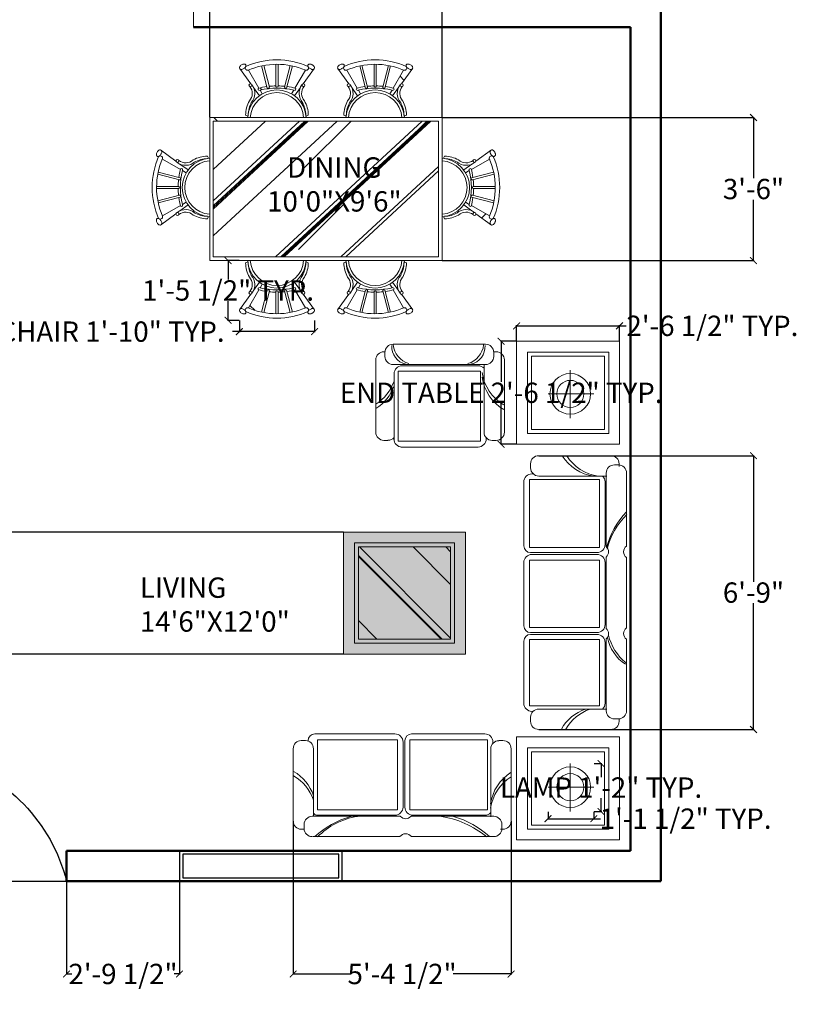
# Model space of a CAD drawing. Units: inches. Extents: x -40 to 418, y 1212 to 1787.
# Tile 2 of 3: x 189 to 418, y 1212 to 1503. Entities that reach past the tile are written whole.
import ezdxf

# ---------------------------------------------------------------- set-up
doc = ezdxf.new("R2010")
doc.units = ezdxf.units.IN
doc.header["$MEASUREMENT"] = 0
for name, color, linetype, lineweight in [('A-ANNO-DIMS', 2, 'Continuous', 18), ('A-AREA-IDEN', 7, 'Continuous', 25), ('A-DOOR', 4, 'Continuous', 25), ('A-FLOR-STRS', 7, 'Continuous', 18), ('A-FURN', 8, 'Continuous', 18), ('A-FURN-PATT', 252, 'Continuous', 9), ('A-GLAZ', 4, 'Continuous', 25), ('A-WALL', 7, 'Continuous', 50)]:
    doc.layers.add(name, color=color, linetype=linetype, lineweight=lineweight)
doc.styles.get("Standard").update_dxf_attribs({"font": 'arial.ttf'})
doc.dimstyles.get("Standard").update_dxf_attribs({"dimtxt": 6, "dimasz": 2, "dimexe": 0.18, "dimexo": 0.0625, "dimgap": 0.09, "dimtad": 0, "dimtih": 1, "dimtoh": 1, "dimdec": 0, "dimzin": 0, "dimdsep": 46, "dimlunit": 4, "dimtxsty": 'Standard', "dimblk": 'ARCHTICK', "dimcen": 0.09, "dimadec": 0, "dimazin": 0, "dimtfac": 1, "dimtdec": 0, "dimtofl": 0, "dimtmove": 0, "dimatfit": 3, "dimldrblk": 'ARCHTICK', "dimfxl": 1, "dimtolj": 1, "dimtzin": 0, "dimarcsym": 0})

# ---------------------------------------------------------------- blocks, each defined once
blk = doc.blocks.new('EREGTHYGUI')
for p, q in [((195.43, 1607.14), (194.43, 1607.14)), ((194.43, 1607.14), (194.43, 1571.14)), ((195.43, 1571.14), (195.43, 1607.14)), ((195.43, 1571.14), (159.43, 1571.14))]:
    blk.add_line(p, q)
blk.add_arc((207.79, 1559.14), 49.82, 105.5486, 166.0653)
blk = doc.blocks.new('CHAIR-DINING')
for p, q in [((2.44, 22.2), (7.04, 18.86)), ((16.3, 20.36), (16.62, 19.71)), ((3.05, 19.5), (8.36, 16.43)), ((8.19, 18.02), (10.6, 16.27)), ((1.67, 15), (8.07, 13.32)), ((1.81, 15.67), (8.31, 13.96)), ((8.97, 16.07), (10.06, 15.44)), ((7.87, 11.44), (1.32, 11.44)), ((7.87, 10.76), (1.32, 10.76)), ((1.67, 7.2), (8.07, 8.88)), ((1.81, 6.54), (8.31, 8.24)), ((8.19, 4.19), (10.6, 5.94)), ((8.97, 6.13), (10.06, 6.76)), ((2.44, 0), (7.04, 3.35)), ((3.03, 2.69), (8.36, 5.78)), ((1.77, 1.96), (1.88, 2.03)), ((16.3, 1.85), (16.62, 2.5))]:
    blk.add_line(p, q)
for centre in [(7.46, 18.93), (7.46, 3.28)]:
    blk.add_circle(centre, 0.429)
for centre, radius, start, end in [((2.48, 20.8), 1.23, 162.4869, 178.6827), ((2.07, 20.81), 0.81, 178.6827, 202.9463), ((3.05, 20.63), 1.82, 149.4208, 162.4869), ((1.71, 20.67), 0.427, 202.9463, 239.4208), ((3.05, 20.63), 1.82, 136.3547, 149.4208), ((2.62, 21.04), 1.23, 120.1589, 136.3547), ((1.67, 21.05), 0.81, 275.8952, 300.1589), ((2.41, 19.76), 0.681, 320.0132, 132.3292), ((2.41, 21.4), 0.81, 95.8952, 120.1589), ((1.46, 21.41), 1.23, 300.1589, 316.3547), ((1.03, 21.82), 1.82, 316.3547, 329.4208), ((1.03, 21.82), 1.82, 329.4208, 342.4869), ((2.02, 21.63), 0.81, 358.6827, 22.9463), ((1.6, 21.64), 1.23, 342.4869, 358.6827), ((16.39, 11.74), 8.62, 90.6047, 119.6593), ((22.82, 11.1), 22.82, 156.3029, 203.6971), ((22.82, 11.1), 21.51, 156.5904, 203.0195), ((1.71, 20.67), 0.427, 239.4208, 275.8952), ((9.91, 21.73), 4.09, 232.0366, 311.5094), ((9.91, 21.73), 3.34, 231.8564, 311.5094), ((17.54, 11.1), 8.65, 93.5658, 266.4342), ((17.54, 11.1), 7.9, 93.9059, 266.0941), ((16.39, 11.74), 7.87, 90.6047, 119.6593), ((28.95, 11.1), 21.27, 164.9077, 171.9728), ((28.95, 11.1), 20.59, 166.0263, 193.9737), ((8.61, 16.29), 0.397, 354.5597, 119.1725), ((28.95, 11.1), 21.27, 173.8131, 179.0879), ((8.03, 13.7), 0.382, 269.2705, 42.4169), ((28.95, 11.1), 21.27, 180.9121, 186.1869), ((7.65, 11.1), 0.405, 303.1978, 56.8022), ((8.03, 8.5), 0.382, 317.5831, 90.7295), ((28.95, 11.1), 21.27, 188.0272, 195.0923), ((8.61, 5.91), 0.397, 240.8275, 5.4403), ((9.91, 0.48), 4.09, 48.4906, 127.9634), ((9.91, 0.48), 3.34, 48.4906, 128.1436), ((16.39, 10.47), 8.62, 240.3407, 269.3953), ((16.39, 10.47), 7.87, 240.3407, 269.3953), ((2.07, 1.39), 0.81, 157.0537, 181.3173), ((2.48, 1.4), 1.23, 181.3173, 197.5131), ((3.05, 1.58), 1.82, 197.5131, 210.5792), ((1.71, 1.54), 0.427, 120.5792, 157.0537), ((3.05, 1.58), 1.82, 210.5792, 223.6453), ((1.71, 1.54), 0.427, 84.1048, 120.5792), ((2.62, 1.17), 1.23, 223.6453, 239.8411), ((1.67, 1.16), 0.81, 59.8411, 84.1048), ((2.41, 2.45), 0.681, 227.6708, 39.9868), ((2.41, 0.81), 0.81, 239.8411, 264.1048), ((1.46, 0.8), 1.23, 43.6453, 59.8411), ((1.03, 0.39), 1.82, 30.5792, 43.6453), ((1.03, 0.39), 1.82, 17.5131, 30.5792), ((1.6, 0.57), 1.23, 1.3173, 17.5131), ((2.02, 0.57), 0.81, 337.0537, 1.3173)]:
    blk.add_arc(centre, radius, start, end)
blk = doc.blocks.new('WIN-48IN')
for points in [[(0, 0), (9, 0), (9, 48), (0, 48)], [(1, 1), (8, 1), (8, 47), (1, 47)]]:
    blk.add_lwpolyline(points, close=True)
blk = doc.blocks.new('TABLE-END-SQUARE')
for p, q in [((30.4, 30.4), (0, 30.4)), ((0, 30.4), (0, 0)), ((30.4, 0), (30.4, 30.4)), ((27.2, 27.2), (3.2, 27.2)), ((3.2, 27.2), (3.2, 3.2)), ((27.2, 3.2), (27.2, 27.2)), ((26, 26), (4.4, 26)), ((4.4, 26), (4.4, 4.4)), ((26, 4.4), (26, 26)), ((3.2, 3.2), (27.2, 3.2)), ((4.4, 4.4), (26, 4.4)), ((0, 0), (30.4, 0))]:
    blk.add_line(p, q)
blk = doc.blocks.new('LAMP-TABLE')
for p, q in [((6.57, 14.12), (6.57, 0)), ((13.54, 7.16), (0, 7.16))]:
    blk.add_line(p, q)
for radius in [6, 4]:
    blk.add_circle((6.57, 7.16), radius)
blk = doc.blocks.new('_ArchTick')
at = {"color": 0, "linetype": 'ByBlock', "const_width": 0.15}
blk.add_lwpolyline([(-0.5, -0.5), (0.5, 0.5)], dxfattribs=at)
blk = doc.blocks.new('*D21')
at = {"layer": 'A-ANNO-DIMS', "color": 0, "lineweight": -2, "transparency": 16777216}
for p, q in [((253.98, 1414.1), (253.98, 1410.66)), ((276.18, 1414.1), (276.18, 1410.66)), ((253.98, 1410.84), (251.98, 1410.84)), ((276.18, 1410.84), (253.98, 1410.84))]:
    blk.add_line(p, q, dxfattribs=at)
at = {"layer": 'Defpoints', "color": 0, "transparency": 16777216}
for p in [(253.98, 1414.17), (276.18, 1414.17), (253.98, 1410.84)]:
    blk.add_point(p, dxfattribs=at)
at = {"layer": 'A-ANNO-DIMS', "color": 0, "lineweight": -2, "transparency": 16777216, "xscale": 2, "yscale": 2, "zscale": 2}
for p, rotation in [((253.98, 1410.84), 179.9999999999912), ((276.18, 1410.84), 359.9999999999912)]:
    blk.add_blockref('_ArchTick', p, dxfattribs=dict(at, rotation=rotation))
at = {"layer": 'A-ANNO-DIMS', "color": 0, "transparency": 16777216, "insert": (201.38, 1410.84), "char_height": 6, "attachment_point": 5}
blk.add_mtext('\\A1;DINING CHAIR 1\'-10" TYP.', dxfattribs=at)
blk = doc.blocks.new('*D22')
at = {"layer": 'A-ANNO-DIMS', "color": 0, "lineweight": -2, "transparency": 16777216}
for p, q in [((253.92, 1431.81), (250.47, 1431.81)), ((250.65, 1431.81), (250.65, 1426.18)), ((250.65, 1414.17), (250.65, 1419.8)), ((253.92, 1414.17), (250.47, 1414.17))]:
    blk.add_line(p, q, dxfattribs=at)
at = {"layer": 'Defpoints', "color": 0, "transparency": 16777216}
for p in [(250.65, 1431.81), (253.98, 1431.81), (253.98, 1414.17)]:
    blk.add_point(p, dxfattribs=at)
at = {"layer": 'A-ANNO-DIMS', "color": 0, "lineweight": -2, "transparency": 16777216, "xscale": 2, "yscale": 2, "zscale": 2}
for p, rotation in [((250.65, 1431.81), 90), ((250.65, 1414.17), 270)]:
    blk.add_blockref('_ArchTick', p, dxfattribs=dict(at, rotation=rotation))
at = {"layer": 'A-ANNO-DIMS', "color": 0, "transparency": 16777216, "insert": (250.65, 1422.99), "char_height": 6, "attachment_point": 5}
blk.add_mtext('\\A1;1\'-5 1/2" TYP.', dxfattribs=at)
blk = doc.blocks.new('*D27')
at = {"layer": 'A-ANNO-DIMS', "color": 0, "lineweight": -2, "transparency": 16777216}
for p, q in [((335.77, 1407.99), (331.09, 1407.99)), ((331.27, 1407.99), (331.27, 1395.98)), ((331.27, 1377.59), (331.27, 1389.6)), ((335.77, 1377.59), (331.09, 1377.59))]:
    blk.add_line(p, q, dxfattribs=at)
at = {"layer": 'Defpoints', "color": 0, "transparency": 16777216}
for p in [(331.27, 1407.99), (335.83, 1407.99), (335.83, 1377.59)]:
    blk.add_point(p, dxfattribs=at)
at = {"layer": 'A-ANNO-DIMS', "color": 0, "lineweight": -2, "transparency": 16777216, "xscale": 2, "yscale": 2, "zscale": 2}
for p, rotation in [((331.27, 1407.99), 90), ((331.27, 1377.59), 270)]:
    blk.add_blockref('_ArchTick', p, dxfattribs=dict(at, rotation=rotation))
at = {"layer": 'A-ANNO-DIMS', "color": 0, "transparency": 16777216, "insert": (331.27, 1392.79), "char_height": 6, "attachment_point": 5}
blk.add_mtext('\\A1;END TABLE 2\'-6 1/2" TYP.', dxfattribs=at)
blk = doc.blocks.new('*D28')
at = {"layer": 'A-ANNO-DIMS', "color": 0, "lineweight": -2, "transparency": 16777216}
for p, q in [((335.83, 1408.05), (335.83, 1412.73)), ((335.83, 1412.55), (366.23, 1412.55)), ((366.23, 1408.05), (366.23, 1412.73)), ((366.23, 1412.55), (368.23, 1412.55))]:
    blk.add_line(p, q, dxfattribs=at)
at = {"layer": 'Defpoints', "color": 0, "transparency": 16777216}
for p in [(366.23, 1412.55), (335.83, 1407.99), (366.23, 1407.99)]:
    blk.add_point(p, dxfattribs=at)
at = {"layer": 'A-ANNO-DIMS', "color": 0, "lineweight": -2, "transparency": 16777216, "xscale": 2, "yscale": 2, "zscale": 2, "rotation": 180}
blk.add_blockref('_ArchTick', (335.83, 1412.55), dxfattribs=at)
at = {"layer": 'A-ANNO-DIMS', "color": 0, "lineweight": -2, "transparency": 16777216, "xscale": 2, "yscale": 2, "zscale": 2}
blk.add_blockref('_ArchTick', (366.23, 1412.55), dxfattribs=at)
at = {"layer": 'A-ANNO-DIMS', "color": 0, "transparency": 16777216, "insert": (393.65, 1412.55), "char_height": 6, "attachment_point": 5}
blk.add_mtext('\\A1;2\'-6 1/2" TYP.', dxfattribs=at)
blk = doc.blocks.new('*D29')
at = {"layer": 'A-ANNO-DIMS', "color": 0, "lineweight": -2, "transparency": 16777216}
for p, q in [((358.72, 1283.36), (360.96, 1283.36)), ((360.78, 1283.36), (360.78, 1279.41)), ((360.78, 1269.24), (360.78, 1273.2)), ((358.72, 1269.24), (360.96, 1269.24))]:
    blk.add_line(p, q, dxfattribs=at)
at = {"layer": 'Defpoints', "color": 0, "transparency": 16777216}
for p in [(358.66, 1283.36), (360.78, 1283.36), (358.66, 1269.24)]:
    blk.add_point(p, dxfattribs=at)
at = {"layer": 'A-ANNO-DIMS', "color": 0, "lineweight": -2, "transparency": 16777216, "xscale": 2, "yscale": 2, "zscale": 2}
for p, rotation in [((360.78, 1283.36), 90), ((360.78, 1269.24), 270)]:
    blk.add_blockref('_ArchTick', p, dxfattribs=dict(at, rotation=rotation))
at = {"layer": 'A-ANNO-DIMS', "color": 0, "transparency": 16777216, "insert": (360.78, 1276.3), "char_height": 6, "attachment_point": 5}
blk.add_mtext('\\A1;LAMP 1\'-2" TYP.', dxfattribs=at)
blk = doc.blocks.new('*D30')
at = {"layer": 'A-ANNO-DIMS', "color": 0, "lineweight": -2, "transparency": 16777216}
for p, q in [((345.12, 1269.18), (345.12, 1266.94)), ((345.12, 1267.12), (358.66, 1267.12)), ((358.66, 1269.18), (358.66, 1266.94)), ((358.66, 1267.12), (360.66, 1267.12))]:
    blk.add_line(p, q, dxfattribs=at)
at = {"layer": 'Defpoints', "color": 0, "transparency": 16777216}
for p in [(345.12, 1269.24), (358.66, 1269.24), (358.66, 1267.12)]:
    blk.add_point(p, dxfattribs=at)
at = {"layer": 'A-ANNO-DIMS', "color": 0, "lineweight": -2, "transparency": 16777216, "xscale": 2, "yscale": 2, "zscale": 2, "rotation": 180}
blk.add_blockref('_ArchTick', (345.12, 1267.12), dxfattribs=at)
at = {"layer": 'A-ANNO-DIMS', "color": 0, "lineweight": -2, "transparency": 16777216, "xscale": 2, "yscale": 2, "zscale": 2}
blk.add_blockref('_ArchTick', (358.66, 1267.12), dxfattribs=at)
at = {"layer": 'A-ANNO-DIMS', "color": 0, "transparency": 16777216, "insert": (385.74, 1267.12), "char_height": 6, "attachment_point": 5}
blk.add_mtext('\\A1;1\'-1 1/2" TYP.', dxfattribs=at)
blk = doc.blocks.new('*D35')
at = {"layer": 'A-ANNO-DIMS', "color": 0, "lineweight": -2, "transparency": 16777216}
for p, q in [((202.93, 1248.57), (202.93, 1221.11)), ((236.31, 1248.57), (236.31, 1221.11)), ((202.93, 1221.29), (204.52, 1221.29)), ((236.31, 1221.29), (234.73, 1221.29))]:
    blk.add_line(p, q, dxfattribs=at)
at = {"layer": 'Defpoints', "color": 0, "transparency": 16777216}
for p in [(202.93, 1248.64), (236.31, 1248.64), (236.31, 1221.29)]:
    blk.add_point(p, dxfattribs=at)
at = {"layer": 'A-ANNO-DIMS', "color": 0, "lineweight": -2, "transparency": 16777216, "xscale": 2, "yscale": 2, "zscale": 2, "rotation": 180}
blk.add_blockref('_ArchTick', (202.93, 1221.29), dxfattribs=at)
at = {"layer": 'A-ANNO-DIMS', "color": 0, "lineweight": -2, "transparency": 16777216, "xscale": 2, "yscale": 2, "zscale": 2}
blk.add_blockref('_ArchTick', (236.31, 1221.29), dxfattribs=at)
at = {"layer": 'A-ANNO-DIMS', "color": 0, "transparency": 16777216, "insert": (219.62, 1221.29), "char_height": 6, "attachment_point": 5}
blk.add_mtext('\\A1;2\'-9 1/2"', dxfattribs=at)
blk = doc.blocks.new('*D39')
at = {"layer": 'A-ANNO-DIMS', "color": 0, "lineweight": -2, "transparency": 16777216}
for p, q in [((245.24, 1474.1), (245.24, 1756.17)), ((245.24, 1755.99), (264.49, 1755.99)), ((313.85, 1755.99), (294.6, 1755.99)), ((313.85, 1474.1), (313.85, 1756.17))]:
    blk.add_line(p, q, dxfattribs=at)
at = {"layer": 'Defpoints', "color": 0, "transparency": 16777216}
for p in [(313.85, 1755.99), (245.24, 1474.03), (313.85, 1474.03)]:
    blk.add_point(p, dxfattribs=at)
at = {"layer": 'A-ANNO-DIMS', "color": 0, "lineweight": -2, "transparency": 16777216, "xscale": 2, "yscale": 2, "zscale": 2, "rotation": 180}
blk.add_blockref('_ArchTick', (245.24, 1755.99), dxfattribs=at)
at = {"layer": 'A-ANNO-DIMS', "color": 0, "lineweight": -2, "transparency": 16777216, "xscale": 2, "yscale": 2, "zscale": 2}
blk.add_blockref('_ArchTick', (313.85, 1755.99), dxfattribs=at)
at = {"layer": 'A-ANNO-DIMS', "color": 0, "transparency": 16777216, "insert": (279.54, 1755.99), "char_height": 6, "attachment_point": 5}
blk.add_mtext('\\A1;5\'-8 1/2"', dxfattribs=at)
blk = doc.blocks.new('*D40')
at = {"layer": 'A-ANNO-DIMS', "color": 0, "lineweight": -2, "transparency": 16777216}
for p, q in [((313.91, 1474.03), (405.96, 1474.03)), ((405.78, 1474.03), (405.78, 1456.08)), ((405.78, 1431.81), (405.78, 1449.77)), ((313.91, 1431.81), (405.96, 1431.81))]:
    blk.add_line(p, q, dxfattribs=at)
at = {"layer": 'Defpoints', "color": 0, "transparency": 16777216}
for p in [(313.85, 1474.03), (405.78, 1474.03), (313.85, 1431.81)]:
    blk.add_point(p, dxfattribs=at)
at = {"layer": 'A-ANNO-DIMS', "color": 0, "lineweight": -2, "transparency": 16777216, "xscale": 2, "yscale": 2, "zscale": 2}
for p, rotation in [((405.78, 1474.03), 90), ((405.78, 1431.81), 270)]:
    blk.add_blockref('_ArchTick', p, dxfattribs=dict(at, rotation=rotation))
at = {"layer": 'A-ANNO-DIMS', "color": 0, "transparency": 16777216, "insert": (405.78, 1452.92), "char_height": 6, "attachment_point": 5}
blk.add_mtext('\\A1;3\'-6"', dxfattribs=at)
blk = doc.blocks.new('*D41')
at = {"layer": 'A-ANNO-DIMS', "color": 0, "lineweight": -2, "transparency": 16777216}
for p, q in [((284.69, 1351.7), (-9.1, 1351.7)), ((-8.92, 1351.7), (-8.92, 1336.86)), ((-8.92, 1315.7), (-8.92, 1330.55)), ((284.69, 1315.7), (-9.1, 1315.7))]:
    blk.add_line(p, q, dxfattribs=at)
at = {"layer": 'Defpoints', "color": 0, "transparency": 16777216}
for p in [(-8.92, 1351.7), (284.75, 1351.7), (284.75, 1315.7)]:
    blk.add_point(p, dxfattribs=at)
at = {"layer": 'A-ANNO-DIMS', "color": 0, "lineweight": -2, "transparency": 16777216, "xscale": 2, "yscale": 2, "zscale": 2}
for p, rotation in [((-8.92, 1351.7), 90), ((-8.92, 1315.7), 270)]:
    blk.add_blockref('_ArchTick', p, dxfattribs=dict(at, rotation=rotation))
at = {"layer": 'A-ANNO-DIMS', "color": 0, "transparency": 16777216, "insert": (-8.92, 1333.7), "char_height": 6, "attachment_point": 5}
blk.add_mtext('\\A1;3\'-0"', dxfattribs=at)
blk = doc.blocks.new('*D42')
at = {"layer": 'A-ANNO-DIMS', "color": 0, "lineweight": -2, "transparency": 16777216}
for p, q in [((342.42, 1374.23), (405.96, 1374.23)), ((405.78, 1374.23), (405.78, 1336.99)), ((405.78, 1293.44), (405.78, 1330.68)), ((342.42, 1293.44), (405.96, 1293.44))]:
    blk.add_line(p, q, dxfattribs=at)
at = {"layer": 'Defpoints', "color": 0, "transparency": 16777216}
for p in [(342.36, 1374.23), (405.78, 1374.23), (342.36, 1293.44)]:
    blk.add_point(p, dxfattribs=at)
at = {"layer": 'A-ANNO-DIMS', "color": 0, "lineweight": -2, "transparency": 16777216, "xscale": 2, "yscale": 2, "zscale": 2}
for p, rotation in [((405.78, 1374.23), 90), ((405.78, 1293.44), 270)]:
    blk.add_blockref('_ArchTick', p, dxfattribs=dict(at, rotation=rotation))
at = {"layer": 'A-ANNO-DIMS', "color": 0, "transparency": 16777216, "insert": (405.78, 1333.83), "char_height": 6, "attachment_point": 5}
blk.add_mtext('\\A1;6\'-9"', dxfattribs=at)
blk = doc.blocks.new('*D43')
at = {"layer": 'A-ANNO-DIMS', "color": 0, "lineweight": -2, "transparency": 16777216}
for p, q in [((269.87, 1266.35), (269.87, 1221.11)), ((334.21, 1266.35), (334.21, 1221.11)), ((269.87, 1221.29), (286.99, 1221.29)), ((334.21, 1221.29), (317.1, 1221.29))]:
    blk.add_line(p, q, dxfattribs=at)
at = {"layer": 'Defpoints', "color": 0, "transparency": 16777216}
for p in [(269.87, 1266.41), (334.21, 1266.41), (334.21, 1221.29)]:
    blk.add_point(p, dxfattribs=at)
at = {"layer": 'A-ANNO-DIMS', "color": 0, "lineweight": -2, "transparency": 16777216, "xscale": 2, "yscale": 2, "zscale": 2, "rotation": 180}
blk.add_blockref('_ArchTick', (269.87, 1221.29), dxfattribs=at)
at = {"layer": 'A-ANNO-DIMS', "color": 0, "lineweight": -2, "transparency": 16777216, "xscale": 2, "yscale": 2, "zscale": 2}
blk.add_blockref('_ArchTick', (334.21, 1221.29), dxfattribs=at)
at = {"layer": 'A-ANNO-DIMS', "color": 0, "transparency": 16777216, "insert": (302.04, 1221.29), "char_height": 6, "attachment_point": 5}
blk.add_mtext('\\A1;5\'-4 1/2"', dxfattribs=at)

msp = doc.modelspace()

# ---------------------------------------------------------------- hatches: boundary and pattern name
at = {"layer": 'A-FURN-PATT'}
h = msp.add_hatch(dxfattribs=at)
h.set_pattern_fill('CROSS', color=256, scale=1.4, angle=315, style=0)
h.set_pattern_definition([(315, (4444.52858, 3949.2683), (0.494974747, -1e-16), [0.175, -0.525]), (45, (4444.52858, 3949.14456), (2e-16, 0.494974747), [0.175, -0.525])])
h.paths.add_polyline_path([(284.75, 1315.7), (320.75, 1315.7), (320.75, 1351.7), (284.75, 1351.7)])
h = msp.add_hatch(dxfattribs=at)
h.set_pattern_fill('AR-RROOF', color=256, scale=20, angle=315, style=0)
h.set_pattern_definition([(315, (4444.529, 3949.268), (45.25483, -16.97056), [300, -40, 100, -20]), (315, (4470.41, 3937.53), (4.6669, 32.95118), [60, -6.6, 120, -15]), (315, (4463.62, 3954.218), (83.014336, -64.063874), [160, -28, 80, -20])])
h.paths.add_polyline_path([(289.15, 1320.1), (316.35, 1320.1), (316.35, 1347.3), (289.15, 1347.3)])

# ---------------------------------------------------------------- linework, layer by layer
at = {"layer": 'A-FLOR-STRS'}
msp.add_line((240.43, 1536.14), (240.43, 1500.64), dxfattribs=at)
at = {"layer": 'A-FURN'}
for p, q in [((301.44, 1486.2), (302.59, 1485.04)), ((260.09, 1482.76), (260.65, 1482.2)), ((296.61, 1482.63), (296.52, 1482.54)), ((297.12, 1483.14), (297.02, 1483.04)), ((245.24, 1431.81), (245.24, 1474.03)), ((245.24, 1474.03), (313.85, 1474.03)), ((246.43, 1474.03), (247.48, 1472.98)), ((313.85, 1474.03), (313.85, 1431.81)), ((282.87, 1472.98), (246.29, 1439.1)), ((274.33, 1472.98), (246.29, 1447.01)), ((273.8, 1472.98), (246.29, 1447.5)), ((271.69, 1472.98), (246.29, 1449.46)), ((273.27, 1472.98), (246.29, 1447.99)), ((261.72, 1472.98), (246.29, 1458.69)), ((246.29, 1432.87), (246.29, 1472.98)), ((246.29, 1472.98), (312.79, 1472.98)), ((307.92, 1472.98), (264.61, 1432.87)), ((309.5, 1472.98), (266.19, 1432.87)), ((310.03, 1472.98), (266.72, 1432.87)), ((310.56, 1472.98), (267.24, 1432.87)), ((286.96, 1472.98), (273.14, 1459.16)), ((309.35, 1472.98), (296.68, 1460.31)), ((312.79, 1472.98), (312.79, 1432.87)), ((312.79, 1459.6), (283.93, 1432.87)), ((312.79, 1458.27), (285.37, 1432.87)), ((285.05, 1448.68), (271.4, 1435.03)), ((326.74, 1445.59), (325.53, 1444.37)), ((312.79, 1432.87), (246.29, 1432.87)), ((313.85, 1431.81), (245.24, 1431.81)), ((257.1, 1418.58), (258.53, 1417.14)), ((326.67, 1407.11), (299.37, 1407.11)), ((296.97, 1404.91), (296.66, 1404.91)), ((296.97, 1404.71), (296.97, 1403.51)), ((329.05, 1404.91), (329.82, 1404.91)), ((329.07, 1404.71), (329.07, 1403.51)), ((294.26, 1381.16), (294.26, 1402.51)), ((326.67, 1401.11), (299.37, 1401.11)), ((302.05, 1400.78), (324.46, 1400.78)), ((326.22, 1381.16), (326.22, 1401.28)), ((332.22, 1381.16), (332.22, 1402.51)), ((299.65, 1398.38), (299.65, 1378.78)), ((300.83, 1399.16), (300.83, 1378.49)), ((325.21, 1399.16), (300.83, 1399.16)), ((325.21, 1378.49), (325.21, 1399.16)), ((297.86, 1378.76), (296.66, 1378.76)), ((299.62, 1379.55), (299.62, 1379.18)), ((300.83, 1378.49), (325.21, 1378.49)), ((326.86, 1379.53), (326.86, 1379.18)), ((328.62, 1378.76), (329.82, 1378.76)), ((301.65, 1376.78), (324.46, 1376.78)), ((339.96, 1370.63), (339.96, 1371.83)), ((342.36, 1374.23), (363.7, 1374.23)), ((365.9, 1371.52), (364.7, 1371.52)), ((366.1, 1371.06), (366.1, 1371.83)), ((340.75, 1368.87), (340.37, 1368.87)), ((362.3, 1347.41), (362.3, 1369.12)), ((368.3, 1347.55), (368.3, 1369.12)), ((337.97, 1347.64), (337.97, 1366.47)), ((339.68, 1347.14), (339.68, 1367.23)), ((339.68, 1367.23), (360.35, 1367.23)), ((342.36, 1368.23), (362.47, 1368.23)), ((360.35, 1367.23), (360.35, 1347.14)), ((361.97, 1348.04), (361.97, 1366.47)), ((320.75, 1351.7), (284.75, 1351.7)), ((284.75, 1351.7), (284.75, 1315.7)), ((320.75, 1315.7), (320.75, 1351.7)), ((317.55, 1348.5), (287.95, 1348.5)), ((287.95, 1348.5), (287.95, 1318.9)), ((317.55, 1318.9), (317.55, 1348.5)), ((316.35, 1347.3), (289.15, 1347.3)), ((289.15, 1347.3), (289.15, 1320.1)), ((316.35, 1320.1), (316.35, 1347.3)), ((360.35, 1347.14), (339.68, 1347.14)), ((359.57, 1345.64), (339.97, 1345.64)), ((337.97, 1324.02), (337.97, 1342.69)), ((339.68, 1323.52), (339.68, 1343.44)), ((339.68, 1343.44), (360.35, 1343.44)), ((359.57, 1345.09), (340.37, 1345.09)), ((360.35, 1343.44), (360.35, 1323.52)), ((361.97, 1324.42), (361.97, 1342.69)), ((362.3, 1323.27), (362.3, 1344.33)), ((368.3, 1323.42), (368.3, 1344.18)), ((360.35, 1323.52), (339.68, 1323.52)), ((359.57, 1322.02), (339.97, 1322.02)), ((289.15, 1320.1), (316.35, 1320.1)), ((337.97, 1319.48), (337.97, 1301.19)), ((360.35, 1319.98), (339.68, 1319.98)), ((339.68, 1319.98), (339.68, 1300.44)), ((359.57, 1321.48), (339.97, 1321.48)), ((360.35, 1300.44), (360.35, 1319.98)), ((362.3, 1298.98), (362.3, 1320.19)), ((368.3, 1298.98), (368.3, 1320.05)), ((287.95, 1318.9), (317.55, 1318.9)), ((361.97, 1319.08), (361.97, 1301.19)), ((284.75, 1315.7), (320.75, 1315.7)), ((339.68, 1300.44), (360.35, 1300.44)), ((340.72, 1298.79), (340.37, 1298.79)), ((342.36, 1299.44), (362.47, 1299.44)), ((339.96, 1297.04), (339.96, 1295.84)), ((365.9, 1296.58), (364.7, 1296.58)), ((366.1, 1296.6), (366.1, 1295.84)), ((342.36, 1293.44), (363.7, 1293.44)), ((273.47, 1290.16), (272.27, 1290.16)), ((274.28, 1290.02), (274.28, 1290.14)), ((276.28, 1292.14), (299.91, 1292.14)), ((277.04, 1269.76), (277.04, 1290.43)), ((277.04, 1290.43), (300.66, 1290.43)), ((300.66, 1290.43), (300.66, 1269.76)), ((302.85, 1270.54), (302.85, 1290.14)), ((304.35, 1269.76), (304.35, 1290.43)), ((304.35, 1290.43), (327.21, 1290.43)), ((304.85, 1292.14), (326.46, 1292.14)), ((327.21, 1290.43), (327.21, 1269.76)), ((330.61, 1290.16), (331.81, 1290.16)), ((269.87, 1287.76), (269.87, 1266.41)), ((275.87, 1287.76), (275.87, 1267.78)), ((302.31, 1270.54), (302.31, 1289.74)), ((328.21, 1287.76), (328.21, 1267.64)), ((328.86, 1289.37), (328.86, 1289.74)), ((334.21, 1287.76), (334.21, 1266.41)), ((300.66, 1269.76), (277.04, 1269.76)), ((327.21, 1269.76), (304.35, 1269.76)), ((275.53, 1267.81), (301.54, 1267.81)), ((277.08, 1268.14), (299.91, 1268.14)), ((304.62, 1267.81), (329.1, 1267.81)), ((305.25, 1268.14), (326.46, 1268.14)), ((273.04, 1264.01), (272.27, 1264.01)), ((273.1, 1264.21), (273.1, 1265.41)), ((331.04, 1264.01), (331.81, 1264.01)), ((331.5, 1264.21), (331.5, 1265.41)), ((275.68, 1261.81), (301.4, 1261.81)), ((304.77, 1261.81), (329.1, 1261.81))]:
    msp.add_line(p, q, dxfattribs=at)
for centre, radius, start, end in [((299.37, 1404.71), 2.4, 90, 180), ((304.41, 1406.5), 5.45, 177.3095, 256.6227), ((305.78, 1407.57), 6.4, 185.3664, 254.1928), ((319.72, 1407.57), 6.4, 285.8072, 354.6336), ((321.09, 1406.5), 5.45, 283.3773, 2.6905), ((326.67, 1404.71), 2.4, 0, 90), ((296.66, 1402.51), 2.4, 90, 180), ((299.37, 1403.51), 2.4, 180, 270), ((326.67, 1403.51), 2.4, 270, 0), ((329.82, 1402.51), 2.4, 0, 90), ((302.05, 1398.38), 2.4, 90, 180), ((324.46, 1398.38), 2.4, 43.0161, 90), ((338.7, 1400.6), 13.19, 188.0636, 239.8898), ((287.23, 1400.6), 13.19, 302.2352, 340.4279), ((287.23, 1399.27), 13.19, 302.2352, 340.4279), ((338.7, 1399.27), 13.19, 188.0636, 239.8898), ((296.66, 1381.16), 2.4, 180, 270), ((328.62, 1381.16), 2.4, 180, 270), ((329.82, 1381.16), 2.4, 270, 0), ((297.86, 1381.19), 2.4, 270, 318.29), ((302.02, 1379.18), 2.4, 180, 270), ((324.46, 1379.18), 2.4, 270, 0), ((342.36, 1371.83), 2.4, 90, 180), ((360.46, 1381.26), 13.19, 212.2352, 261.9364), ((361.79, 1381.26), 13.19, 212.2352, 261.9364), ((364.7, 1369.12), 2.4, 90, 180), ((363.7, 1371.83), 2.4, 0, 90), ((365.9, 1369.12), 2.4, 0, 90), ((340.37, 1366.47), 2.4, 90, 180), ((342.38, 1370.63), 2.4, 180, 270), ((359.57, 1366.47), 2.4, 0, 46.9839), ((386.4, 1340.63), 24.87, 136.7033, 164.9108), ((383.38, 1341.65), 21.36, 134.5575, 166.454), ((339.97, 1347.64), 2, 180, 270), ((359.57, 1348.04), 2.4, 270, 0), ((360.92, 1345.87), 2.07, 311.9207, 48.0793), ((369.5, 1345.87), 2.07, 125.5086, 234.4914), ((340.37, 1342.69), 2.4, 90, 180), ((359.57, 1342.69), 2.4, 0, 90), ((339.97, 1324.02), 2, 180, 270), ((359.57, 1324.42), 2.4, 270, 0), ((360.92, 1321.73), 2.07, 311.9207, 48.0793), ((369.5, 1321.73), 2.07, 125.5086, 234.4914), ((339.97, 1319.48), 2, 90, 180), ((359.57, 1319.08), 2.4, 0, 90), ((375.15, 1323.25), 12.8, 192.0984, 235.7661), ((377.66, 1324.94), 15.16, 193.8701, 231.2301), ((340.37, 1301.19), 2.4, 180, 270), ((342.36, 1297.04), 2.4, 90, 180), ((360.46, 1286.95), 13.19, 108.8232, 149.8898), ((361.79, 1286.95), 13.19, 108.8232, 149.8898), ((359.57, 1301.19), 2.4, 313.0161, 0), ((364.7, 1298.98), 2.4, 180, 270), ((365.9, 1298.98), 2.4, 270, 0), ((342.36, 1295.84), 2.4, 180, 270), ((363.7, 1295.84), 2.4, 270, 0), ((272.27, 1287.76), 2.4, 90, 180), ((273.47, 1287.76), 2.4, 0, 90), ((276.28, 1290.14), 2, 90, 180), ((299.91, 1289.74), 2.4, 0, 90), ((304.85, 1290.14), 2, 90, 180), ((326.46, 1289.74), 2.4, 0, 90), ((330.61, 1287.73), 2.4, 90, 180), ((331.81, 1287.76), 2.4, 0, 90), ((263.39, 1269.65), 13.19, 18.8232, 59.8898), ((263.39, 1268.32), 13.19, 18.8232, 59.8898), ((341.24, 1269.65), 13.19, 122.2352, 171.9364), ((341.24, 1268.32), 13.19, 122.2352, 171.9364), ((299.91, 1270.54), 2.4, 270, 0), ((305.25, 1270.54), 2.4, 180, 270), ((275.5, 1265.41), 2.4, 90, 180), ((277.03, 1269.5), 1.36, 211.7185, 272.2999), ((293.32, 1243.71), 24.87, 105.0892, 133.2967), ((292.29, 1246.73), 21.36, 99.3588, 135.4425), ((303.08, 1269.19), 2.07, 221.9207, 318.0793), ((309.37, 1240.4), 27.68, 50.3908, 82.0603), ((310.77, 1243.71), 24.87, 46.7033, 74.9108), ((326.46, 1270.54), 2.4, 270, 316.9839), ((329.1, 1265.41), 2.4, 0, 90), ((272.27, 1266.41), 2.4, 180, 270), ((275.5, 1264.21), 2.4, 180, 270), ((329.1, 1264.21), 2.4, 270, 0), ((331.81, 1266.41), 2.4, 270, 0), ((303.08, 1260.61), 2.07, 35.5086, 144.4914)]:
    msp.add_arc(centre, radius, start, end, dxfattribs=at)
at = {"layer": 'A-WALL'}
for p, q in [((378.43, 1728.64), (378.43, 1248.64)), ((240.43, 1500.64), (369.43, 1500.64)), ((369.43, 1500.64), (369.43, 1257.64)), ((369.43, 1257.64), (202.93, 1257.64)), ((202.93, 1248.64), (202.93, 1257.64)), ((378.43, 1248.64), (202.93, 1248.64))]:
    msp.add_line(p, q, dxfattribs=at)

# ---------------------------------------------------------------- block references
at = {"layer": 'A-DOOR', "xscale": -1}
msp.add_blockref('EREGTHYGUI', (362.37, -322.5), dxfattribs=at)
at = {"layer": 'A-FURN', "extrusion": (0, 0, -1), "zscale": -1}
for p, rotation in [((-276.18, 1491.04), 269.9999999999915), ((-305.18, 1491.04), 269.9999999999893)]:
    msp.add_blockref('CHAIR-DINING', p, dxfattribs=dict(at, rotation=rotation))
at = {"layer": 'A-FURN'}
for name, p in [('CHAIR-DINING', (228.23, 1442.27)), ('TABLE-END-SQUARE', (335.83, 1377.59)), ('LAMP-TABLE', (345.12, 1385.3)), ('LAMP-TABLE', (345.12, 1269.24))]:
    msp.add_blockref(name, p, dxfattribs=at)
at = {"layer": 'A-FURN', "extrusion": (0, 0, -1), "zscale": -1}
msp.add_blockref('CHAIR-DINING', (-330.85, 1442.27), dxfattribs=at)
at = {"layer": 'A-FURN'}
for name, p, rotation in [('CHAIR-DINING', (276.18, 1414.81), 89.99999999999122), ('CHAIR-DINING', (305.18, 1414.81), 89.99999999998919), ('TABLE-END-SQUARE', (366.23, 1260.84), 90.00000000000063)]:
    msp.add_blockref(name, p, dxfattribs=dict(at, rotation=rotation))
at = {"layer": 'A-GLAZ', "rotation": 269.9999999999991}
msp.add_blockref('WIN-48IN', (236.31, 1257.64), dxfattribs=at)

# ---------------------------------------------------------------- texts
at = {"layer": 'A-AREA-IDEN', "char_height": 6, "attachment_point": 1}
for s, width, insert in [('\\pxqc;DINING^J10\'0"X9\'6"', 144.321, (209.87, 1462.27)), ('LIVING\\P14\'6"X12\'0"', 167.6365, (224.6, 1338.29))]:
    msp.add_mtext_dynamic_manual_height_columns(s, width=width, gutter_width=30, heights=[0], dxfattribs=dict(at, insert=insert))

# ---------------------------------------------------------------- dimensions: what is measured, and where the dimension line sits
at = {"layer": 'A-ANNO-DIMS'}
for base, p1, p2, picture, middle in [((313.85, 1755.99), (245.24, 1474.03), (313.85, 1474.03), '*D39', (279.54, 1755.99)), ((334.21, 1221.29), (269.87, 1266.41), (334.21, 1266.41), '*D43', (302.04, 1221.29)), ((236.31, 1221.29), (202.93, 1248.64), (236.31, 1248.64), '*D35', (219.62, 1221.29))]:
    dim = msp.add_linear_dim(base=base, p1=p1, p2=p2, dimstyle='Standard', override={"dimdec": 1, "dimlfac": 1, "dimrnd": 0, "dimzin": 1, "dimdsep": 46, "dimlunit": 4, "dimfrac": 2}, dxfattribs=at)
    dim.commit()
    dim.dimension.update_dxf_attribs({"geometry": picture, "text_midpoint": middle})
for base, p1, p2, picture, middle in [((405.78, 1474.03), (313.85, 1431.81), (313.85, 1474.03), '*D40', (405.78, 1452.92)), ((405.78, 1374.23), (342.36, 1293.44), (342.36, 1374.23), '*D42', (405.78, 1333.83)), ((-8.92, 1351.7), (284.75, 1315.7), (284.75, 1351.7), '*D41', (-8.92, 1333.7))]:
    dim = msp.add_linear_dim(base=base, p1=p1, p2=p2, angle=90, dimstyle='Standard', override={"dimdec": 1, "dimlfac": 1, "dimrnd": 0, "dimzin": 1, "dimdsep": 46, "dimlunit": 4, "dimfrac": 2}, dxfattribs=at)
    dim.commit()
    dim.dimension.update_dxf_attribs({"geometry": picture, "text_midpoint": middle})
for base, p1, p2, angle, text, picture, middle in [((250.65, 1431.81), (253.98, 1414.17), (253.98, 1431.81), 90, '<> TYP.', '*D22', (250.65, 1422.99)), ((253.98, 1410.84), (276.18, 1414.17), (253.98, 1414.17), 180, 'DINING CHAIR <> TYP.', '*D21', (201.38, 1410.84)), ((331.27, 1407.99), (335.83, 1377.59), (335.83, 1407.99), 90, 'END TABLE <> TYP.', '*D27', (331.27, 1392.79)), ((360.78, 1283.36), (358.66, 1269.24), (358.66, 1283.36), 90, 'LAMP <> TYP.', '*D29', (360.78, 1276.3))]:
    dim = msp.add_linear_dim(base=base, p1=p1, p2=p2, angle=angle, text=text, dimstyle='Standard', override={"dimdec": 1, "dimlfac": 1, "dimrnd": 0, "dimzin": 1, "dimdsep": 46, "dimlunit": 4, "dimfrac": 2}, dxfattribs=at)
    dim.commit()
    dim.dimension.update_dxf_attribs({"geometry": picture, "text_midpoint": middle})
for base, p1, p2, picture, middle in [((366.23, 1412.55), (335.83, 1407.99), (366.23, 1407.99), '*D28', (393.65, 1412.55)), ((358.66, 1267.12), (345.12, 1269.24), (358.66, 1269.24), '*D30', (385.74, 1267.12))]:
    dim = msp.add_linear_dim(base=base, p1=p1, p2=p2, text='<> TYP.', dimstyle='Standard', override={"dimdec": 1, "dimlfac": 1, "dimrnd": 0, "dimzin": 1, "dimdsep": 46, "dimlunit": 4, "dimfrac": 2}, dxfattribs=at)
    dim.commit()
    dim.dimension.update_dxf_attribs({"geometry": picture, "text_midpoint": middle})

doc.saveas('drawing.dxf')
